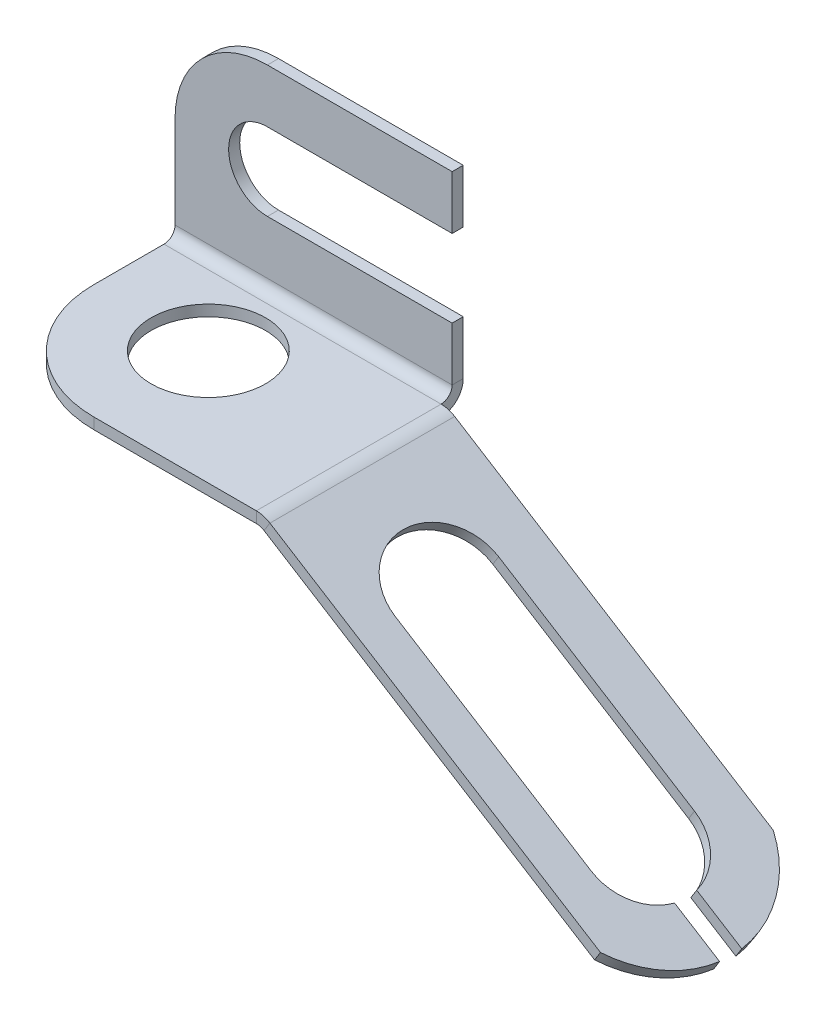
ISO-10303-21;
HEADER;
FILE_DESCRIPTION(('STEP AP214'),'2;1');
FILE_NAME('part.step','',(''),(''),'','','');
FILE_SCHEMA(('AUTOMOTIVE_DESIGN { 1 0 10303 214 1 1 1 1 }'));
ENDSEC;
DATA;
#1=APPLICATION_CONTEXT('core data for automotive mechanical design processes');
#2=APPLICATION_PROTOCOL_DEFINITION('international standard','automotive_design',2000,#1);
#3=PRODUCT_CONTEXT('',#1,'mechanical');
#4=PRODUCT('Part','Part','',(#3));
#5=PRODUCT_RELATED_PRODUCT_CATEGORY('part','',(#4));
#6=PRODUCT_DEFINITION_FORMATION('','',#4);
#7=PRODUCT_DEFINITION_CONTEXT('part definition',#1,'design');
#8=PRODUCT_DEFINITION('design','',#6,#7);
#9=PRODUCT_DEFINITION_SHAPE('','',#8);
#10=(LENGTH_UNIT() NAMED_UNIT(*) SI_UNIT(.MILLI.,.METRE.));
#11=(NAMED_UNIT(*) PLANE_ANGLE_UNIT() SI_UNIT($,.RADIAN.));
#12=(NAMED_UNIT(*) SI_UNIT($,.STERADIAN.) SOLID_ANGLE_UNIT());
#13=UNCERTAINTY_MEASURE_WITH_UNIT(LENGTH_MEASURE(1.E-05),#10,'distance_accuracy_value','');
#14=(GEOMETRIC_REPRESENTATION_CONTEXT(3) GLOBAL_UNCERTAINTY_ASSIGNED_CONTEXT((#13)) GLOBAL_UNIT_ASSIGNED_CONTEXT((#10,
#11,#12)) REPRESENTATION_CONTEXT('',''));
#15=CARTESIAN_POINT('',(0.,0.,0.));
#16=DIRECTION('',(0.,0.,1.));
#17=DIRECTION('',(1.,0.,0.));
#18=AXIS2_PLACEMENT_3D('',#15,#16,#17);
#19=CARTESIAN_POINT('',(0.,0.,0.002000000000002));
#20=DIRECTION('',(0.,-1.,0.));
#21=DIRECTION('',(0.,0.,-1.));
#22=AXIS2_PLACEMENT_3D('',#19,#20,#21);
#23=PLANE('',#22);
#24=CARTESIAN_POINT('',(0.,0.,0.));
#25=DIRECTION('',(0.,1.,0.));
#26=DIRECTION('',(0.,0.,1.));
#27=AXIS2_PLACEMENT_3D('',#24,#25,#26);
#28=CIRCLE('',#27,7.874);
#29=CARTESIAN_POINT('',(0.,0.,7.874));
#30=VERTEX_POINT('',#29);
#31=EDGE_CURVE('E347',#30,#30,#28,.T.);
#32=ORIENTED_EDGE('',*,*,#31,.F.);
#33=EDGE_LOOP('',(#32));
#34=FACE_BOUND('',#33,.T.);
#35=DIRECTION('',(1.,0.,0.));
#36=VECTOR('',#35,1.);
#37=CARTESIAN_POINT('',(0.,0.,15.75));
#38=LINE('',#37,#36);
#39=CARTESIAN_POINT('',(0.,0.,15.75));
#40=VERTEX_POINT('',#39);
#41=CARTESIAN_POINT('',(22.352,0.,15.75));
#42=VERTEX_POINT('',#41);
#43=EDGE_CURVE('E54',#40,#42,#38,.T.);
#44=ORIENTED_EDGE('',*,*,#43,.T.);
#45=DIRECTION('',(0.,0.,-1.));
#46=VECTOR('',#45,1.);
#47=CARTESIAN_POINT('',(22.352,0.,0.002000000000002));
#48=LINE('',#47,#46);
#49=CARTESIAN_POINT('',(22.352,0.,-9.65312139112702));
#50=VERTEX_POINT('',#49);
#51=EDGE_CURVE('E58',#42,#50,#48,.T.);
#52=ORIENTED_EDGE('',*,*,#51,.T.);
#53=DIRECTION('',(1.,0.,0.));
#54=VECTOR('',#53,1.);
#55=CARTESIAN_POINT('',(0.,0.,-9.65312139112702));
#56=LINE('',#55,#54);
#57=CARTESIAN_POINT('',(-15.748,0.,-9.65312139112702));
#58=VERTEX_POINT('',#57);
#59=EDGE_CURVE('E328',#58,#50,#56,.T.);
#60=ORIENTED_EDGE('',*,*,#59,.F.);
#61=DIRECTION('',(0.,0.,1.));
#62=VECTOR('',#61,1.);
#63=CARTESIAN_POINT('',(-15.748,0.,-25.94));
#64=LINE('',#63,#62);
#65=CARTESIAN_POINT('',(-15.748,0.,0.00200000000000489));
#66=VERTEX_POINT('',#65);
#67=EDGE_CURVE('E342',#58,#66,#64,.T.);
#68=ORIENTED_EDGE('',*,*,#67,.T.);
#69=CARTESIAN_POINT('',(0.,0.,0.002000000000002));
#70=DIRECTION('',(0.,1.,0.));
#71=DIRECTION('',(0.,0.,-1.));
#72=AXIS2_PLACEMENT_3D('',#69,#70,#71);
#73=CIRCLE('',#72,15.748);
#74=EDGE_CURVE('E339',#66,#40,#73,.T.);
#75=ORIENTED_EDGE('',*,*,#74,.T.);
#76=EDGE_LOOP('',(#44,#52,#60,#68,#75));
#77=FACE_BOUND('',#76,.T.);
#78=ADVANCED_FACE('F51',(#34,#77),#23,.F.);
#79=CARTESIAN_POINT('',(0.,-11.719678608873,-11.1731213911271));
#80=DIRECTION('',(0.,0.,-1.));
#81=DIRECTION('',(0.,1.,0.));
#82=AXIS2_PLACEMENT_3D('',#79,#80,#81);
#83=PLANE('',#82);
#84=DIRECTION('',(0.,-1.,0.));
#85=VECTOR('',#84,1.);
#86=CARTESIAN_POINT('',(-15.748,14.222321391127,-11.173121391127));
#87=LINE('',#86,#85);
#88=CARTESIAN_POINT('',(-15.748,14.222321391127,-11.173121391127));
#89=VERTEX_POINT('',#88);
#90=CARTESIAN_POINT('',(-15.748,1.52,-11.173121391127));
#91=VERTEX_POINT('',#90);
#92=EDGE_CURVE('E398',#89,#91,#87,.T.);
#93=ORIENTED_EDGE('',*,*,#92,.T.);
#94=DIRECTION('',(1.,0.,0.));
#95=VECTOR('',#94,1.);
#96=CARTESIAN_POINT('',(0.,1.52,-11.173121391127));
#97=LINE('',#96,#95);
#98=CARTESIAN_POINT('',(22.352,1.52,-11.173121391127));
#99=VERTEX_POINT('',#98);
#100=EDGE_CURVE('E420',#91,#99,#97,.T.);
#101=ORIENTED_EDGE('',*,*,#100,.T.);
#102=DIRECTION('',(0.,1.,0.));
#103=VECTOR('',#102,1.);
#104=CARTESIAN_POINT('',(22.352,8.88832139112702,-11.173121391127));
#105=LINE('',#104,#103);
#106=CARTESIAN_POINT('',(22.352,8.88832139112702,-11.173121391127));
#107=VERTEX_POINT('',#106);
#108=EDGE_CURVE('E331',#99,#107,#105,.T.);
#109=ORIENTED_EDGE('',*,*,#108,.T.);
#110=DIRECTION('',(-1.,0.,0.));
#111=VECTOR('',#110,1.);
#112=CARTESIAN_POINT('',(22.352,8.88832139112702,-11.173121391127));
#113=LINE('',#112,#111);
#114=CARTESIAN_POINT('',(-3.04799999999999,8.88832139112702,-11.173121391127));
#115=VERTEX_POINT('',#114);
#116=EDGE_CURVE('E377',#107,#115,#113,.T.);
#117=ORIENTED_EDGE('',*,*,#116,.T.);
#118=CARTESIAN_POINT('',(-3.048,14.222321391127,-11.173121391127));
#119=DIRECTION('',(0.,0.,-1.));
#120=DIRECTION('',(0.,1.,0.));
#121=AXIS2_PLACEMENT_3D('',#118,#119,#120);
#122=CIRCLE('',#121,5.334);
#123=CARTESIAN_POINT('',(-3.048,19.556321391127,-11.173121391127));
#124=VERTEX_POINT('',#123);
#125=EDGE_CURVE('E382',#115,#124,#122,.T.);
#126=ORIENTED_EDGE('',*,*,#125,.T.);
#127=DIRECTION('',(1.,0.,0.));
#128=VECTOR('',#127,1.);
#129=CARTESIAN_POINT('',(-3.048,19.556321391127,-11.173121391127));
#130=LINE('',#129,#128);
#131=CARTESIAN_POINT('',(22.352,19.556321391127,-11.173121391127));
#132=VERTEX_POINT('',#131);
#133=EDGE_CURVE('E381',#124,#132,#130,.T.);
#134=ORIENTED_EDGE('',*,*,#133,.T.);
#135=DIRECTION('',(0.,1.,0.));
#136=VECTOR('',#135,1.);
#137=CARTESIAN_POINT('',(22.352,19.556321391127,-11.173121391127));
#138=LINE('',#137,#136);
#139=CARTESIAN_POINT('',(22.352,26.922321391127,-11.1731213911269));
#140=VERTEX_POINT('',#139);
#141=EDGE_CURVE('E390',#132,#140,#138,.T.);
#142=ORIENTED_EDGE('',*,*,#141,.T.);
#143=DIRECTION('',(-1.,0.,0.));
#144=VECTOR('',#143,1.);
#145=CARTESIAN_POINT('',(22.352,26.922321391127,-11.1731213911269));
#146=LINE('',#145,#144);
#147=CARTESIAN_POINT('',(-3.048,26.922321391127,-11.1731213911269));
#148=VERTEX_POINT('',#147);
#149=EDGE_CURVE('E388',#140,#148,#146,.T.);
#150=ORIENTED_EDGE('',*,*,#149,.T.);
#151=CARTESIAN_POINT('',(-3.048,14.222321391127,-11.173121391127));
#152=DIRECTION('',(0.,0.,1.));
#153=DIRECTION('',(0.,-1.,0.));
#154=AXIS2_PLACEMENT_3D('',#151,#152,#153);
#155=CIRCLE('',#154,12.7);
#156=EDGE_CURVE('E392',#148,#89,#155,.T.);
#157=ORIENTED_EDGE('',*,*,#156,.T.);
#158=EDGE_LOOP('',(#93,#101,#109,#117,#126,#134,#142,#150,#157));
#159=FACE_BOUND('',#158,.T.);
#160=ADVANCED_FACE('F518',(#159),#83,.F.);
#161=CARTESIAN_POINT('',(22.352,8.88832139112703,-12.697121391127));
#162=DIRECTION('',(1.,0.,0.));
#163=DIRECTION('',(0.,1.,0.));
#164=AXIS2_PLACEMENT_3D('',#161,#162,#163);
#165=PLANE('',#164);
#166=DIRECTION('',(0.,0.,1.));
#167=VECTOR('',#166,1.);
#168=CARTESIAN_POINT('',(22.352,1.52000000000001,-12.697121391127));
#169=LINE('',#168,#167);
#170=CARTESIAN_POINT('',(22.352,1.52000000000001,-12.697121391127));
#171=VERTEX_POINT('',#170);
#172=EDGE_CURVE('E414',#171,#99,#169,.T.);
#173=ORIENTED_EDGE('',*,*,#172,.F.);
#174=DIRECTION('',(0.,1.,0.));
#175=VECTOR('',#174,1.);
#176=CARTESIAN_POINT('',(22.352,8.88832139112703,-12.697121391127));
#177=LINE('',#176,#175);
#178=CARTESIAN_POINT('',(22.352,8.88832139112703,-12.697121391127));
#179=VERTEX_POINT('',#178);
#180=EDGE_CURVE('E365',#171,#179,#177,.T.);
#181=ORIENTED_EDGE('',*,*,#180,.T.);
#182=DIRECTION('',(0.,0.,1.));
#183=VECTOR('',#182,1.);
#184=CARTESIAN_POINT('',(22.352,8.88832139112703,-12.697121391127));
#185=LINE('',#184,#183);
#186=EDGE_CURVE('E408',#179,#107,#185,.T.);
#187=ORIENTED_EDGE('',*,*,#186,.T.);
#188=ORIENTED_EDGE('',*,*,#108,.F.);
#189=EDGE_LOOP('',(#173,#181,#187,#188));
#190=FACE_BOUND('',#189,.T.);
#191=ADVANCED_FACE('F530',(#190),#165,.T.);
#192=CARTESIAN_POINT('',(-15.748,14.222321391127,-12.697121391127));
#193=DIRECTION('',(-1.,0.,0.));
#194=DIRECTION('',(0.,-1.,0.));
#195=AXIS2_PLACEMENT_3D('',#192,#193,#194);
#196=PLANE('',#195);
#197=DIRECTION('',(0.,0.,-1.));
#198=VECTOR('',#197,1.);
#199=CARTESIAN_POINT('',(-15.748,1.52000000000001,-12.697121391127));
#200=LINE('',#199,#198);
#201=CARTESIAN_POINT('',(-15.748,1.52000000000001,-12.697121391127));
#202=VERTEX_POINT('',#201);
#203=EDGE_CURVE('E419',#91,#202,#200,.T.);
#204=ORIENTED_EDGE('',*,*,#203,.F.);
#205=ORIENTED_EDGE('',*,*,#92,.F.);
#206=DIRECTION('',(0.,0.,1.));
#207=VECTOR('',#206,1.);
#208=CARTESIAN_POINT('',(-15.748,14.222321391127,-12.697121391127));
#209=LINE('',#208,#207);
#210=CARTESIAN_POINT('',(-15.748,14.222321391127,-12.697121391127));
#211=VERTEX_POINT('',#210);
#212=EDGE_CURVE('E400',#211,#89,#209,.T.);
#213=ORIENTED_EDGE('',*,*,#212,.F.);
#214=DIRECTION('',(0.,-1.,0.));
#215=VECTOR('',#214,1.);
#216=CARTESIAN_POINT('',(-15.748,14.222321391127,-12.697121391127));
#217=LINE('',#216,#215);
#218=EDGE_CURVE('E380',#211,#202,#217,.T.);
#219=ORIENTED_EDGE('',*,*,#218,.T.);
#220=EDGE_LOOP('',(#204,#205,#213,#219));
#221=FACE_BOUND('',#220,.T.);
#222=ADVANCED_FACE('F504',(#221),#196,.T.);
#223=CARTESIAN_POINT('',(-3.048,14.222321391127,-12.697121391127));
#224=DIRECTION('',(0.,0.,1.));
#225=DIRECTION('',(0.,-1.,0.));
#226=AXIS2_PLACEMENT_3D('',#223,#224,#225);
#227=CYLINDRICAL_SURFACE('',#226,12.7);
#228=ORIENTED_EDGE('',*,*,#156,.F.);
#229=DIRECTION('',(0.,0.,1.));
#230=VECTOR('',#229,1.);
#231=CARTESIAN_POINT('',(-3.048,26.922321391127,-12.6971213911269));
#232=LINE('',#231,#230);
#233=CARTESIAN_POINT('',(-3.048,26.922321391127,-12.6971213911269));
#234=VERTEX_POINT('',#233);
#235=EDGE_CURVE('E397',#234,#148,#232,.T.);
#236=ORIENTED_EDGE('',*,*,#235,.F.);
#237=CARTESIAN_POINT('',(-3.048,14.222321391127,-12.697121391127));
#238=DIRECTION('',(0.,0.,1.));
#239=DIRECTION('',(0.,-1.,0.));
#240=AXIS2_PLACEMENT_3D('',#237,#238,#239);
#241=CIRCLE('',#240,12.7);
#242=EDGE_CURVE('E372',#234,#211,#241,.T.);
#243=ORIENTED_EDGE('',*,*,#242,.T.);
#244=ORIENTED_EDGE('',*,*,#212,.T.);
#245=EDGE_LOOP('',(#228,#236,#243,#244));
#246=FACE_BOUND('',#245,.T.);
#247=ADVANCED_FACE('F537',(#246),#227,.T.);
#248=CARTESIAN_POINT('',(22.352,26.922321391127,-12.6971213911269));
#249=DIRECTION('',(0.,1.,0.));
#250=DIRECTION('',(-1.,0.,0.));
#251=AXIS2_PLACEMENT_3D('',#248,#249,#250);
#252=PLANE('',#251);
#253=ORIENTED_EDGE('',*,*,#149,.F.);
#254=DIRECTION('',(0.,0.,1.));
#255=VECTOR('',#254,1.);
#256=CARTESIAN_POINT('',(22.352,26.922321391127,-12.6971213911269));
#257=LINE('',#256,#255);
#258=CARTESIAN_POINT('',(22.352,26.922321391127,-12.6971213911269));
#259=VERTEX_POINT('',#258);
#260=EDGE_CURVE('E405',#259,#140,#257,.T.);
#261=ORIENTED_EDGE('',*,*,#260,.F.);
#262=DIRECTION('',(-1.,0.,0.));
#263=VECTOR('',#262,1.);
#264=CARTESIAN_POINT('',(22.352,26.922321391127,-12.6971213911269));
#265=LINE('',#264,#263);
#266=EDGE_CURVE('E371',#259,#234,#265,.T.);
#267=ORIENTED_EDGE('',*,*,#266,.T.);
#268=ORIENTED_EDGE('',*,*,#235,.T.);
#269=EDGE_LOOP('',(#253,#261,#267,#268));
#270=FACE_BOUND('',#269,.T.);
#271=ADVANCED_FACE('F559',(#270),#252,.T.);
#272=CARTESIAN_POINT('',(22.352,19.556321391127,-12.697121391127));
#273=DIRECTION('',(1.,0.,0.));
#274=DIRECTION('',(0.,1.,0.));
#275=AXIS2_PLACEMENT_3D('',#272,#273,#274);
#276=PLANE('',#275);
#277=ORIENTED_EDGE('',*,*,#141,.F.);
#278=DIRECTION('',(0.,0.,1.));
#279=VECTOR('',#278,1.);
#280=CARTESIAN_POINT('',(22.352,19.556321391127,-12.697121391127));
#281=LINE('',#280,#279);
#282=CARTESIAN_POINT('',(22.352,19.556321391127,-12.697121391127));
#283=VERTEX_POINT('',#282);
#284=EDGE_CURVE('E404',#283,#132,#281,.T.);
#285=ORIENTED_EDGE('',*,*,#284,.F.);
#286=DIRECTION('',(0.,1.,0.));
#287=VECTOR('',#286,1.);
#288=CARTESIAN_POINT('',(22.352,19.556321391127,-12.697121391127));
#289=LINE('',#288,#287);
#290=EDGE_CURVE('E368',#283,#259,#289,.T.);
#291=ORIENTED_EDGE('',*,*,#290,.T.);
#292=ORIENTED_EDGE('',*,*,#260,.T.);
#293=EDGE_LOOP('',(#277,#285,#291,#292));
#294=FACE_BOUND('',#293,.T.);
#295=ADVANCED_FACE('F554',(#294),#276,.T.);
#296=CARTESIAN_POINT('',(-3.048,19.556321391127,-12.697121391127));
#297=DIRECTION('',(0.,-1.,0.));
#298=DIRECTION('',(1.,0.,0.));
#299=AXIS2_PLACEMENT_3D('',#296,#297,#298);
#300=PLANE('',#299);
#301=ORIENTED_EDGE('',*,*,#133,.F.);
#302=DIRECTION('',(0.,0.,1.));
#303=VECTOR('',#302,1.);
#304=CARTESIAN_POINT('',(-3.048,19.556321391127,-12.697121391127));
#305=LINE('',#304,#303);
#306=CARTESIAN_POINT('',(-3.048,19.556321391127,-12.697121391127));
#307=VERTEX_POINT('',#306);
#308=EDGE_CURVE('E407',#307,#124,#305,.T.);
#309=ORIENTED_EDGE('',*,*,#308,.F.);
#310=DIRECTION('',(1.,0.,0.));
#311=VECTOR('',#310,1.);
#312=CARTESIAN_POINT('',(-3.048,19.556321391127,-12.697121391127));
#313=LINE('',#312,#311);
#314=EDGE_CURVE('E362',#307,#283,#313,.T.);
#315=ORIENTED_EDGE('',*,*,#314,.T.);
#316=ORIENTED_EDGE('',*,*,#284,.T.);
#317=EDGE_LOOP('',(#301,#309,#315,#316));
#318=FACE_BOUND('',#317,.T.);
#319=ADVANCED_FACE('F553',(#318),#300,.T.);
#320=CARTESIAN_POINT('',(-3.048,14.222321391127,-12.697121391127));
#321=DIRECTION('',(0.,0.,1.));
#322=DIRECTION('',(0.,-1.,0.));
#323=AXIS2_PLACEMENT_3D('',#320,#321,#322);
#324=CYLINDRICAL_SURFACE('',#323,5.334);
#325=ORIENTED_EDGE('',*,*,#125,.F.);
#326=DIRECTION('',(0.,0.,1.));
#327=VECTOR('',#326,1.);
#328=CARTESIAN_POINT('',(-3.04799999999999,8.88832139112703,-12.697121391127));
#329=LINE('',#328,#327);
#330=CARTESIAN_POINT('',(-3.04799999999999,8.88832139112703,-12.697121391127));
#331=VERTEX_POINT('',#330);
#332=EDGE_CURVE('E409',#331,#115,#329,.T.);
#333=ORIENTED_EDGE('',*,*,#332,.F.);
#334=CARTESIAN_POINT('',(-3.048,14.222321391127,-12.697121391127));
#335=DIRECTION('',(0.,0.,-1.));
#336=DIRECTION('',(0.,1.,0.));
#337=AXIS2_PLACEMENT_3D('',#334,#335,#336);
#338=CIRCLE('',#337,5.334);
#339=EDGE_CURVE('E363',#331,#307,#338,.T.);
#340=ORIENTED_EDGE('',*,*,#339,.T.);
#341=ORIENTED_EDGE('',*,*,#308,.T.);
#342=EDGE_LOOP('',(#325,#333,#340,#341));
#343=FACE_BOUND('',#342,.T.);
#344=ADVANCED_FACE('F550',(#343),#324,.F.);
#345=CARTESIAN_POINT('',(22.352,8.88832139112703,-12.697121391127));
#346=DIRECTION('',(0.,1.,0.));
#347=DIRECTION('',(-1.,0.,0.));
#348=AXIS2_PLACEMENT_3D('',#345,#346,#347);
#349=PLANE('',#348);
#350=ORIENTED_EDGE('',*,*,#116,.F.);
#351=ORIENTED_EDGE('',*,*,#186,.F.);
#352=DIRECTION('',(-1.,0.,0.));
#353=VECTOR('',#352,1.);
#354=CARTESIAN_POINT('',(22.352,8.88832139112703,-12.697121391127));
#355=LINE('',#354,#353);
#356=EDGE_CURVE('E356',#179,#331,#355,.T.);
#357=ORIENTED_EDGE('',*,*,#356,.T.);
#358=ORIENTED_EDGE('',*,*,#332,.T.);
#359=EDGE_LOOP('',(#350,#351,#357,#358));
#360=FACE_BOUND('',#359,.T.);
#361=ADVANCED_FACE('F543',(#360),#349,.T.);
#362=CARTESIAN_POINT('',(0.,-11.719678608873,-12.6971213911271));
#363=DIRECTION('',(0.,0.,-1.));
#364=DIRECTION('',(0.,1.,0.));
#365=AXIS2_PLACEMENT_3D('',#362,#363,#364);
#366=PLANE('',#365);
#367=DIRECTION('',(1.,0.,0.));
#368=VECTOR('',#367,1.);
#369=CARTESIAN_POINT('',(0.,1.52000000000001,-12.697121391127));
#370=LINE('',#369,#368);
#371=EDGE_CURVE('E399',#202,#171,#370,.T.);
#372=ORIENTED_EDGE('',*,*,#371,.F.);
#373=ORIENTED_EDGE('',*,*,#218,.F.);
#374=ORIENTED_EDGE('',*,*,#242,.F.);
#375=ORIENTED_EDGE('',*,*,#266,.F.);
#376=ORIENTED_EDGE('',*,*,#290,.F.);
#377=ORIENTED_EDGE('',*,*,#314,.F.);
#378=ORIENTED_EDGE('',*,*,#339,.F.);
#379=ORIENTED_EDGE('',*,*,#356,.F.);
#380=ORIENTED_EDGE('',*,*,#180,.F.);
#381=EDGE_LOOP('',(#372,#373,#374,#375,#376,#377,#378,#379,#380));
#382=FACE_BOUND('',#381,.T.);
#383=ADVANCED_FACE('F499',(#382),#366,.T.);
#384=CARTESIAN_POINT('',(0.,-1.524,0.002000000000002));
#385=DIRECTION('',(0.,1.,0.));
#386=DIRECTION('',(0.,0.,1.));
#387=AXIS2_PLACEMENT_3D('',#384,#385,#386);
#388=CYLINDRICAL_SURFACE('',#387,15.748);
#389=ORIENTED_EDGE('',*,*,#74,.F.);
#390=DIRECTION('',(0.,1.,0.));
#391=VECTOR('',#390,1.);
#392=CARTESIAN_POINT('',(-15.748,-1.524,0.00200000000000489));
#393=LINE('',#392,#391);
#394=CARTESIAN_POINT('',(-15.748,-1.524,0.00200000000000489));
#395=VERTEX_POINT('',#394);
#396=EDGE_CURVE('E326',#395,#66,#393,.T.);
#397=ORIENTED_EDGE('',*,*,#396,.F.);
#398=CARTESIAN_POINT('',(0.,-1.524,0.002000000000002));
#399=DIRECTION('',(0.,1.,0.));
#400=DIRECTION('',(0.,0.,-1.));
#401=AXIS2_PLACEMENT_3D('',#398,#399,#400);
#402=CIRCLE('',#401,15.748);
#403=CARTESIAN_POINT('',(0.,-1.524,15.75));
#404=VERTEX_POINT('',#403);
#405=EDGE_CURVE('E352',#395,#404,#402,.T.);
#406=ORIENTED_EDGE('',*,*,#405,.T.);
#407=DIRECTION('',(0.,1.,0.));
#408=VECTOR('',#407,1.);
#409=CARTESIAN_POINT('',(0.,-1.524,15.75));
#410=LINE('',#409,#408);
#411=EDGE_CURVE('E355',#404,#40,#410,.T.);
#412=ORIENTED_EDGE('',*,*,#411,.T.);
#413=EDGE_LOOP('',(#389,#397,#406,#412));
#414=FACE_BOUND('',#413,.T.);
#415=ADVANCED_FACE('F542',(#414),#388,.T.);
#416=CARTESIAN_POINT('',(0.,-1.524,15.75));
#417=DIRECTION('',(0.,0.,1.));
#418=DIRECTION('',(1.,0.,0.));
#419=AXIS2_PLACEMENT_3D('',#416,#417,#418);
#420=PLANE('',#419);
#421=DIRECTION('',(0.,-1.,0.));
#422=VECTOR('',#421,1.);
#423=CARTESIAN_POINT('',(22.352,-1.524,15.75));
#424=LINE('',#423,#422);
#425=CARTESIAN_POINT('',(22.352,-1.524,15.75));
#426=VERTEX_POINT('',#425);
#427=EDGE_CURVE('E12',#42,#426,#424,.T.);
#428=ORIENTED_EDGE('',*,*,#427,.F.);
#429=ORIENTED_EDGE('',*,*,#43,.F.);
#430=ORIENTED_EDGE('',*,*,#411,.F.);
#431=DIRECTION('',(1.,0.,0.));
#432=VECTOR('',#431,1.);
#433=CARTESIAN_POINT('',(0.,-1.524,15.75));
#434=LINE('',#433,#432);
#435=EDGE_CURVE('E351',#404,#426,#434,.T.);
#436=ORIENTED_EDGE('',*,*,#435,.T.);
#437=EDGE_LOOP('',(#428,#429,#430,#436));
#438=FACE_BOUND('',#437,.T.);
#439=ADVANCED_FACE('F52',(#438),#420,.T.);
#440=CARTESIAN_POINT('',(0.,-1.524,0.));
#441=DIRECTION('',(0.,1.,0.));
#442=DIRECTION('',(0.,0.,1.));
#443=AXIS2_PLACEMENT_3D('',#440,#441,#442);
#444=CYLINDRICAL_SURFACE('',#443,7.874);
#445=CARTESIAN_POINT('',(0.,-1.524,0.));
#446=DIRECTION('',(0.,1.,0.));
#447=DIRECTION('',(0.,0.,1.));
#448=AXIS2_PLACEMENT_3D('',#445,#446,#447);
#449=CIRCLE('',#448,7.874);
#450=CARTESIAN_POINT('',(0.,-1.524,7.874));
#451=VERTEX_POINT('',#450);
#452=EDGE_CURVE('E343',#451,#451,#449,.T.);
#453=CARTESIAN_POINT('',(0.,-1.524,7.874));
#454=CARTESIAN_POINT('',(0.,-1.508125,7.874));
#455=CARTESIAN_POINT('',(0.,-1.49225,7.874));
#456=CARTESIAN_POINT('',(0.,-1.4605,7.874));
#457=CARTESIAN_POINT('',(0.,-1.444625,7.874));
#458=CARTESIAN_POINT('',(0.,-1.412875,7.874));
#459=CARTESIAN_POINT('',(0.,-1.397,7.874));
#460=CARTESIAN_POINT('',(0.,-1.36525,7.874));
#461=CARTESIAN_POINT('',(0.,-1.349375,7.874));
#462=CARTESIAN_POINT('',(0.,-1.317625,7.874));
#463=CARTESIAN_POINT('',(0.,-1.30175,7.874));
#464=CARTESIAN_POINT('',(0.,-1.27,7.874));
#465=CARTESIAN_POINT('',(0.,-1.254125,7.874));
#466=CARTESIAN_POINT('',(0.,-1.222375,7.874));
#467=CARTESIAN_POINT('',(0.,-1.2065,7.874));
#468=CARTESIAN_POINT('',(0.,-1.17475,7.874));
#469=CARTESIAN_POINT('',(0.,-1.158875,7.874));
#470=CARTESIAN_POINT('',(0.,-1.127125,7.874));
#471=CARTESIAN_POINT('',(0.,-1.11125,7.874));
#472=CARTESIAN_POINT('',(0.,-1.0795,7.874));
#473=CARTESIAN_POINT('',(0.,-1.063625,7.874));
#474=CARTESIAN_POINT('',(0.,-1.031875,7.874));
#475=CARTESIAN_POINT('',(0.,-1.016,7.874));
#476=CARTESIAN_POINT('',(0.,-0.98425,7.874));
#477=CARTESIAN_POINT('',(0.,-0.968375,7.874));
#478=CARTESIAN_POINT('',(0.,-0.936625,7.874));
#479=CARTESIAN_POINT('',(0.,-0.92075,7.874));
#480=CARTESIAN_POINT('',(0.,-0.889,7.874));
#481=CARTESIAN_POINT('',(0.,-0.873125,7.874));
#482=CARTESIAN_POINT('',(0.,-0.841375,7.874));
#483=CARTESIAN_POINT('',(0.,-0.8255,7.874));
#484=CARTESIAN_POINT('',(0.,-0.79375,7.874));
#485=CARTESIAN_POINT('',(0.,-0.777875,7.874));
#486=CARTESIAN_POINT('',(0.,-0.746125,7.874));
#487=CARTESIAN_POINT('',(0.,-0.73025,7.874));
#488=CARTESIAN_POINT('',(0.,-0.6985,7.874));
#489=CARTESIAN_POINT('',(0.,-0.682625,7.874));
#490=CARTESIAN_POINT('',(0.,-0.650875,7.874));
#491=CARTESIAN_POINT('',(0.,-0.635,7.874));
#492=CARTESIAN_POINT('',(0.,-0.60325,7.874));
#493=CARTESIAN_POINT('',(0.,-0.587375,7.874));
#494=CARTESIAN_POINT('',(0.,-0.555625,7.874));
#495=CARTESIAN_POINT('',(0.,-0.53975,7.874));
#496=CARTESIAN_POINT('',(0.,-0.508,7.874));
#497=CARTESIAN_POINT('',(0.,-0.492125,7.874));
#498=CARTESIAN_POINT('',(0.,-0.460375,7.874));
#499=CARTESIAN_POINT('',(0.,-0.4445,7.874));
#500=CARTESIAN_POINT('',(0.,-0.41275,7.874));
#501=CARTESIAN_POINT('',(0.,-0.396875,7.874));
#502=CARTESIAN_POINT('',(0.,-0.365125,7.874));
#503=CARTESIAN_POINT('',(0.,-0.34925,7.874));
#504=CARTESIAN_POINT('',(0.,-0.3175,7.874));
#505=CARTESIAN_POINT('',(0.,-0.301625,7.874));
#506=CARTESIAN_POINT('',(0.,-0.269875,7.874));
#507=CARTESIAN_POINT('',(0.,-0.254,7.874));
#508=CARTESIAN_POINT('',(0.,-0.22225,7.874));
#509=CARTESIAN_POINT('',(0.,-0.206375,7.874));
#510=CARTESIAN_POINT('',(0.,-0.174625,7.874));
#511=CARTESIAN_POINT('',(0.,-0.15875,7.874));
#512=CARTESIAN_POINT('',(0.,-0.127,7.874));
#513=CARTESIAN_POINT('',(0.,-0.111125,7.874));
#514=CARTESIAN_POINT('',(0.,-0.079375,7.874));
#515=CARTESIAN_POINT('',(0.,-0.0635,7.874));
#516=CARTESIAN_POINT('',(0.,-0.0317499999999999,7.874));
#517=CARTESIAN_POINT('',(0.,-0.015875,7.874));
#518=CARTESIAN_POINT('',(0.,0.,7.874));
#519=B_SPLINE_CURVE_WITH_KNOTS('',3,(#453,#454,#455,#456,#457,#458,#459,#460,#461,#462,#463,
#464,#465,#466,#467,#468,#469,#470,#471,#472,#473,#474,#475,#476,#477,#478,#479,#480,#481,#482,
#483,#484,#485,#486,#487,#488,#489,#490,#491,#492,#493,#494,#495,#496,#497,#498,#499,#500,#501,
#502,#503,#504,#505,#506,#507,#508,#509,#510,#511,#512,#513,#514,#515,#516,#517,#518),
.UNSPECIFIED.,.F.,.F.,(4,2,2,2,2,2,2,2,2,2,2,2,2,2,2,2,2,2,2,2,2,2,2,2,2,2,2,2,2,2,2,2,4),(0.,
0.0476250000000001,0.0952500000000001,0.142875,0.1905,0.238125,0.28575,0.333375,0.381,0.428625,
0.47625,0.523875,0.5715,0.619125,0.66675,0.714375,0.762,0.809625,0.85725,0.904875,0.9525,
1.000125,1.04775,1.095375,1.143,1.190625,1.23825,1.285875,1.3335,1.381125,1.42875,1.476375,
1.524),.UNSPECIFIED.);
#520=EDGE_CURVE('BSEAM534',#451,#30,#519,.T.);
#521=ORIENTED_EDGE('',*,*,#452,.F.);
#522=ORIENTED_EDGE('',*,*,#31,.T.);
#523=ORIENTED_EDGE('',*,*,#520,.T.);
#524=ORIENTED_EDGE('',*,*,#520,.F.);
#525=EDGE_LOOP('',(#521,#523,#522,#524));
#526=FACE_BOUND('',#525,.T.);
#527=ADVANCED_FACE('F534',(#526),#444,.F.);
#528=CARTESIAN_POINT('',(0.,-1.524,0.002000000000002));
#529=DIRECTION('',(0.,-1.,0.));
#530=DIRECTION('',(0.,0.,-1.));
#531=AXIS2_PLACEMENT_3D('',#528,#529,#530);
#532=PLANE('',#531);
#533=DIRECTION('',(0.,0.,-1.));
#534=VECTOR('',#533,1.);
#535=CARTESIAN_POINT('',(22.352,-1.524,0.002000000000002));
#536=LINE('',#535,#534);
#537=CARTESIAN_POINT('',(22.352,-1.524,-9.65312139112702));
#538=VERTEX_POINT('',#537);
#539=EDGE_CURVE('E421',#426,#538,#536,.T.);
#540=ORIENTED_EDGE('',*,*,#539,.F.);
#541=ORIENTED_EDGE('',*,*,#435,.F.);
#542=ORIENTED_EDGE('',*,*,#405,.F.);
#543=DIRECTION('',(0.,0.,1.));
#544=VECTOR('',#543,1.);
#545=CARTESIAN_POINT('',(-15.748,-1.524,-25.94));
#546=LINE('',#545,#544);
#547=CARTESIAN_POINT('',(-15.748,-1.524,-9.65312139112702));
#548=VERTEX_POINT('',#547);
#549=EDGE_CURVE('E334',#548,#395,#546,.T.);
#550=ORIENTED_EDGE('',*,*,#549,.F.);
#551=DIRECTION('',(1.,0.,0.));
#552=VECTOR('',#551,1.);
#553=CARTESIAN_POINT('',(0.,-1.524,-9.65312139112702));
#554=LINE('',#553,#552);
#555=EDGE_CURVE('E344',#548,#538,#554,.T.);
#556=ORIENTED_EDGE('',*,*,#555,.T.);
#557=EDGE_LOOP('',(#540,#541,#542,#550,#556));
#558=FACE_BOUND('',#557,.T.);
#559=ORIENTED_EDGE('',*,*,#452,.T.);
#560=EDGE_LOOP('',(#559));
#561=FACE_BOUND('',#560,.T.);
#562=ADVANCED_FACE('F439',(#558,#561),#532,.T.);
#563=CARTESIAN_POINT('',(-15.748,-1.524,-25.94));
#564=DIRECTION('',(-1.,0.,0.));
#565=DIRECTION('',(0.,0.,1.));
#566=AXIS2_PLACEMENT_3D('',#563,#564,#565);
#567=PLANE('',#566);
#568=ORIENTED_EDGE('',*,*,#67,.F.);
#569=DIRECTION('',(0.,-1.,0.));
#570=VECTOR('',#569,1.);
#571=CARTESIAN_POINT('',(-15.748,-1.524,-9.65312139112702));
#572=LINE('',#571,#570);
#573=EDGE_CURVE('E337',#58,#548,#572,.T.);
#574=ORIENTED_EDGE('',*,*,#573,.T.);
#575=ORIENTED_EDGE('',*,*,#549,.T.);
#576=ORIENTED_EDGE('',*,*,#396,.T.);
#577=EDGE_LOOP('',(#568,#574,#575,#576));
#578=FACE_BOUND('',#577,.T.);
#579=ADVANCED_FACE('F517',(#578),#567,.T.);
#580=CARTESIAN_POINT('',(-15.748,1.52,-9.65312139112702));
#581=DIRECTION('',(-1.,0.,0.));
#582=DIRECTION('',(0.,0.,1.));
#583=AXIS2_PLACEMENT_3D('',#580,#581,#582);
#584=PLANE('',#583);
#585=ORIENTED_EDGE('',*,*,#573,.F.);
#586=CARTESIAN_POINT('',(-15.748,1.52,-9.65312139112702));
#587=DIRECTION('',(1.,0.,0.));
#588=DIRECTION('',(0.,0.,-1.));
#589=AXIS2_PLACEMENT_3D('',#586,#587,#588);
#590=CIRCLE('',#589,1.52);
#591=EDGE_CURVE('E314',#58,#91,#590,.T.);
#592=ORIENTED_EDGE('',*,*,#591,.T.);
#593=ORIENTED_EDGE('',*,*,#203,.T.);
#594=CARTESIAN_POINT('',(-15.748,1.52,-9.65312139112702));
#595=DIRECTION('',(1.,0.,0.));
#596=DIRECTION('',(0.,0.,1.));
#597=AXIS2_PLACEMENT_3D('',#594,#595,#596);
#598=CIRCLE('',#597,3.044);
#599=EDGE_CURVE('E318',#548,#202,#598,.T.);
#600=ORIENTED_EDGE('',*,*,#599,.F.);
#601=EDGE_LOOP('',(#585,#592,#593,#600));
#602=FACE_BOUND('',#601,.T.);
#603=ADVANCED_FACE('F508',(#602),#584,.T.);
#604=CARTESIAN_POINT('',(22.352,1.52,-9.65312139112702));
#605=DIRECTION('',(1.,0.,0.));
#606=DIRECTION('',(0.,0.,-1.));
#607=AXIS2_PLACEMENT_3D('',#604,#605,#606);
#608=PLANE('',#607);
#609=CARTESIAN_POINT('',(22.352,1.52,-9.65312139112702));
#610=DIRECTION('',(1.,0.,0.));
#611=DIRECTION('',(0.,0.,-1.));
#612=AXIS2_PLACEMENT_3D('',#609,#610,#611);
#613=CIRCLE('',#612,1.52);
#614=EDGE_CURVE('E72',#99,#50,#613,.F.);
#615=ORIENTED_EDGE('',*,*,#614,.T.);
#616=DIRECTION('',(0.,1.,0.));
#617=VECTOR('',#616,1.);
#618=CARTESIAN_POINT('',(22.352,-1.524,-9.65312139112702));
#619=LINE('',#618,#617);
#620=EDGE_CURVE('E431',#538,#50,#619,.T.);
#621=ORIENTED_EDGE('',*,*,#620,.F.);
#622=CARTESIAN_POINT('',(22.352,1.52,-9.65312139112702));
#623=DIRECTION('',(-1.,0.,0.));
#624=DIRECTION('',(0.,0.,-1.));
#625=AXIS2_PLACEMENT_3D('',#622,#623,#624);
#626=CIRCLE('',#625,3.044);
#627=EDGE_CURVE('E324',#171,#538,#626,.T.);
#628=ORIENTED_EDGE('',*,*,#627,.F.);
#629=ORIENTED_EDGE('',*,*,#172,.T.);
#630=EDGE_LOOP('',(#615,#621,#628,#629));
#631=FACE_BOUND('',#630,.T.);
#632=ADVANCED_FACE('F491',(#631),#608,.T.);
#633=CARTESIAN_POINT('',(-34.9965851755296,1.52,-9.65312139112702));
#634=DIRECTION('',(1.,0.,0.));
#635=DIRECTION('',(0.,0.,-1.));
#636=AXIS2_PLACEMENT_3D('',#633,#634,#635);
#637=CYLINDRICAL_SURFACE('',#636,3.044);
#638=ORIENTED_EDGE('',*,*,#371,.T.);
#639=ORIENTED_EDGE('',*,*,#627,.T.);
#640=ORIENTED_EDGE('',*,*,#555,.F.);
#641=ORIENTED_EDGE('',*,*,#599,.T.);
#642=EDGE_LOOP('',(#638,#639,#640,#641));
#643=FACE_BOUND('',#642,.T.);
#644=ADVANCED_FACE('F492',(#643),#637,.T.);
#645=CARTESIAN_POINT('',(-34.9965851755296,1.52,-9.65312139112702));
#646=DIRECTION('',(1.,0.,0.));
#647=DIRECTION('',(0.,0.,-1.));
#648=AXIS2_PLACEMENT_3D('',#645,#646,#647);
#649=CYLINDRICAL_SURFACE('',#648,1.52);
#650=ORIENTED_EDGE('',*,*,#100,.F.);
#651=ORIENTED_EDGE('',*,*,#591,.F.);
#652=ORIENTED_EDGE('',*,*,#59,.T.);
#653=ORIENTED_EDGE('',*,*,#614,.F.);
#654=EDGE_LOOP('',(#650,#651,#652,#653));
#655=FACE_BOUND('',#654,.T.);
#656=ADVANCED_FACE('F514',(#655),#649,.F.);
#657=CARTESIAN_POINT('',(22.352,-3.524,15.75));
#658=DIRECTION('',(0.,0.,-1.));
#659=DIRECTION('',(-1.,0.,0.));
#660=AXIS2_PLACEMENT_3D('',#657,#658,#659);
#661=PLANE('',#660);
#662=DIRECTION('',(-0.529919264233206,-0.848048096156425,0.));
#663=VECTOR('',#662,1.);
#664=CARTESIAN_POINT('',(23.4118385284664,-1.82790380768715,15.75));
#665=LINE('',#664,#663);
#666=CARTESIAN_POINT('',(24.2194354871578,-0.535478509144757,15.75));
#667=VERTEX_POINT('',#666);
#668=CARTESIAN_POINT('',(23.4118385284664,-1.82790380768715,15.75));
#669=VERTEX_POINT('',#668);
#670=EDGE_CURVE('E232',#667,#669,#665,.T.);
#671=ORIENTED_EDGE('',*,*,#670,.F.);
#672=CARTESIAN_POINT('',(22.352,-3.524,15.75));
#673=DIRECTION('',(0.,0.,1.));
#674=DIRECTION('',(1.,0.,0.));
#675=AXIS2_PLACEMENT_3D('',#672,#673,#674);
#676=CIRCLE('',#675,3.524);
#677=EDGE_CURVE('E250',#667,#42,#676,.T.);
#678=ORIENTED_EDGE('',*,*,#677,.T.);
#679=ORIENTED_EDGE('',*,*,#427,.T.);
#680=CARTESIAN_POINT('',(22.352,-3.524,15.75));
#681=DIRECTION('',(0.,0.,1.));
#682=DIRECTION('',(-1.,0.,0.));
#683=AXIS2_PLACEMENT_3D('',#680,#681,#682);
#684=CIRCLE('',#683,2.);
#685=EDGE_CURVE('E308',#669,#426,#684,.T.);
#686=ORIENTED_EDGE('',*,*,#685,.F.);
#687=EDGE_LOOP('',(#671,#678,#679,#686));
#688=FACE_BOUND('',#687,.T.);
#689=ADVANCED_FACE('F450',(#688),#661,.F.);
#690=CARTESIAN_POINT('',(22.352,-3.524,-9.65312139112702));
#691=DIRECTION('',(0.,0.,1.));
#692=DIRECTION('',(1.,0.,0.));
#693=AXIS2_PLACEMENT_3D('',#690,#691,#692);
#694=PLANE('',#693);
#695=CARTESIAN_POINT('',(22.352,-3.524,-9.65312139112701));
#696=DIRECTION('',(0.,0.,1.));
#697=DIRECTION('',(1.,0.,0.));
#698=AXIS2_PLACEMENT_3D('',#695,#696,#697);
#699=CIRCLE('',#698,3.524);
#700=CARTESIAN_POINT('',(24.2194354871578,-0.535478509144757,-9.65312139112702));
#701=VERTEX_POINT('',#700);
#702=EDGE_CURVE('E315',#50,#701,#699,.F.);
#703=ORIENTED_EDGE('',*,*,#702,.T.);
#704=DIRECTION('',(0.529919264233206,0.848048096156425,0.));
#705=VECTOR('',#704,1.);
#706=CARTESIAN_POINT('',(23.4118385284664,-1.82790380768715,-9.65312139112702));
#707=LINE('',#706,#705);
#708=CARTESIAN_POINT('',(23.4118385284664,-1.82790380768715,-9.65312139112702));
#709=VERTEX_POINT('',#708);
#710=EDGE_CURVE('E466',#709,#701,#707,.T.);
#711=ORIENTED_EDGE('',*,*,#710,.F.);
#712=CARTESIAN_POINT('',(22.352,-3.524,-9.65312139112702));
#713=DIRECTION('',(0.,0.,-1.));
#714=DIRECTION('',(1.,0.,0.));
#715=AXIS2_PLACEMENT_3D('',#712,#713,#714);
#716=CIRCLE('',#715,2.);
#717=EDGE_CURVE('E311',#538,#709,#716,.T.);
#718=ORIENTED_EDGE('',*,*,#717,.F.);
#719=ORIENTED_EDGE('',*,*,#620,.T.);
#720=EDGE_LOOP('',(#703,#711,#718,#719));
#721=FACE_BOUND('',#720,.T.);
#722=ADVANCED_FACE('F493',(#721),#694,.F.);
#723=CARTESIAN_POINT('',(22.352,-3.524,-22.4470650422621));
#724=DIRECTION('',(0.,0.,1.));
#725=DIRECTION('',(1.,0.,0.));
#726=AXIS2_PLACEMENT_3D('',#723,#724,#725);
#727=CYLINDRICAL_SURFACE('',#726,2.);
#728=ORIENTED_EDGE('',*,*,#539,.T.);
#729=ORIENTED_EDGE('',*,*,#717,.T.);
#730=DIRECTION('',(0.,0.,-1.));
#731=VECTOR('',#730,1.);
#732=CARTESIAN_POINT('',(23.4118385284664,-1.82790380768715,0.002000000000002));
#733=LINE('',#732,#731);
#734=EDGE_CURVE('E269',#669,#709,#733,.T.);
#735=ORIENTED_EDGE('',*,*,#734,.F.);
#736=ORIENTED_EDGE('',*,*,#685,.T.);
#737=EDGE_LOOP('',(#728,#729,#735,#736));
#738=FACE_BOUND('',#737,.T.);
#739=ADVANCED_FACE('F446',(#738),#727,.F.);
#740=CARTESIAN_POINT('',(22.352,-3.524,-22.4470650422621));
#741=DIRECTION('',(0.,0.,1.));
#742=DIRECTION('',(1.,0.,0.));
#743=AXIS2_PLACEMENT_3D('',#740,#741,#742);
#744=CYLINDRICAL_SURFACE('',#743,3.524);
#745=ORIENTED_EDGE('',*,*,#51,.F.);
#746=ORIENTED_EDGE('',*,*,#677,.F.);
#747=DIRECTION('',(0.,0.,-1.));
#748=VECTOR('',#747,1.);
#749=CARTESIAN_POINT('',(24.2194354871578,-0.535478509144757,0.002000000000002));
#750=LINE('',#749,#748);
#751=EDGE_CURVE('E259',#667,#701,#750,.T.);
#752=ORIENTED_EDGE('',*,*,#751,.T.);
#753=ORIENTED_EDGE('',*,*,#702,.F.);
#754=EDGE_LOOP('',(#745,#746,#752,#753));
#755=FACE_BOUND('',#754,.T.);
#756=ADVANCED_FACE('F489',(#755),#744,.T.);
#757=CARTESIAN_POINT('',(62.4767570027001,-26.2383740970723,3.55));
#758=DIRECTION('',(0.529919264233206,0.848048096156425,0.));
#759=DIRECTION('',(0.,0.,1.));
#760=AXIS2_PLACEMENT_3D('',#757,#758,#759);
#761=CYLINDRICAL_SURFACE('',#760,14.3346893367871);
#762=DIRECTION('',(0.529919264233206,0.848048096156425,0.));
#763=VECTOR('',#762,1.);
#764=CARTESIAN_POINT('',(70.0727696433476,-40.9796057398259,5.074));
#765=LINE('',#764,#763);
#766=CARTESIAN_POINT('',(74.5643653269883,-33.7915500768041,5.074));
#767=VERTEX_POINT('',#766);
#768=CARTESIAN_POINT('',(75.3719622856797,-32.4991247782617,5.074));
#769=VERTEX_POINT('',#768);
#770=EDGE_CURVE('E254',#767,#769,#765,.T.);
#771=ORIENTED_EDGE('',*,*,#770,.T.);
#772=CARTESIAN_POINT('',(63.2843539613915,-24.9459487985299,3.55));
#773=DIRECTION('',(0.529919264233206,0.848048096156425,0.));
#774=DIRECTION('',(0.,0.,1.));
#775=AXIS2_PLACEMENT_3D('',#772,#773,#774);
#776=CIRCLE('',#775,14.3346893367871);
#777=CARTESIAN_POINT('',(69.6669128063745,-28.9342142075176,15.75));
#778=VERTEX_POINT('',#777);
#779=EDGE_CURVE('E246',#778,#769,#776,.T.);
#780=ORIENTED_EDGE('',*,*,#779,.F.);
#781=DIRECTION('',(0.529919264233206,0.848048096156425,0.));
#782=VECTOR('',#781,1.);
#783=CARTESIAN_POINT('',(68.859315847683,-30.22663950606,15.75));
#784=LINE('',#783,#782);
#785=CARTESIAN_POINT('',(68.859315847683,-30.22663950606,15.75));
#786=VERTEX_POINT('',#785);
#787=EDGE_CURVE('E235',#786,#778,#784,.T.);
#788=ORIENTED_EDGE('',*,*,#787,.F.);
#789=CARTESIAN_POINT('',(62.4767570027001,-26.2383740970723,3.55));
#790=DIRECTION('',(0.529919264233206,0.848048096156425,0.));
#791=DIRECTION('',(0.,0.,1.));
#792=AXIS2_PLACEMENT_3D('',#789,#790,#791);
#793=CIRCLE('',#792,14.3346893367871);
#794=EDGE_CURVE('E242',#786,#767,#793,.T.);
#795=ORIENTED_EDGE('',*,*,#794,.T.);
#796=EDGE_LOOP('',(#771,#780,#788,#795));
#797=FACE_BOUND('',#796,.T.);
#798=ADVANCED_FACE('F243',(#797),#761,.T.);
#799=CARTESIAN_POINT('',(63.8763780343853,-37.1076705309573,5.074));
#800=DIRECTION('',(0.,0.,1.));
#801=DIRECTION('',(0.848048096156425,-0.529919264233206,0.));
#802=AXIS2_PLACEMENT_3D('',#799,#800,#801);
#803=PLANE('',#802);
#804=DIRECTION('',(-0.848048096156425,0.529919264233206,0.));
#805=VECTOR('',#804,1.);
#806=CARTESIAN_POINT('',(3.14807543888309,10.834300701345,5.074));
#807=LINE('',#806,#805);
#808=CARTESIAN_POINT('',(68.367973718026,-29.9196148679354,5.074));
#809=VERTEX_POINT('',#808);
#810=EDGE_CURVE('E255',#767,#809,#807,.T.);
#811=ORIENTED_EDGE('',*,*,#810,.T.);
#812=DIRECTION('',(0.529919264233206,0.848048096156425,0.));
#813=VECTOR('',#812,1.);
#814=CARTESIAN_POINT('',(68.367973718026,-29.9196148679354,5.074));
#815=LINE('',#814,#813);
#816=CARTESIAN_POINT('',(69.1755706767174,-28.627189569393,5.074));
#817=VERTEX_POINT('',#816);
#818=EDGE_CURVE('E285',#817,#809,#815,.F.);
#819=ORIENTED_EDGE('',*,*,#818,.F.);
#820=DIRECTION('',(0.848048096156425,-0.529919264233206,0.));
#821=VECTOR('',#820,1.);
#822=CARTESIAN_POINT('',(69.1755706767174,-28.627189569393,5.074));
#823=LINE('',#822,#821);
#824=EDGE_CURVE('E257',#817,#769,#823,.T.);
#825=ORIENTED_EDGE('',*,*,#824,.T.);
#826=ORIENTED_EDGE('',*,*,#770,.F.);
#827=EDGE_LOOP('',(#811,#819,#825,#826));
#828=FACE_BOUND('',#827,.T.);
#829=ADVANCED_FACE('F617',(#828),#803,.F.);
#830=CARTESIAN_POINT('',(62.4767570027001,-26.2383740970723,3.55));
#831=DIRECTION('',(0.529919264233206,0.848048096156425,0.));
#832=DIRECTION('',(0.,0.,1.));
#833=AXIS2_PLACEMENT_3D('',#830,#831,#832);
#834=CYLINDRICAL_SURFACE('',#833,7.112);
#835=CARTESIAN_POINT('',(63.2843539613915,-24.9459487985299,3.55));
#836=DIRECTION('',(0.529919264233206,0.848048096156425,0.));
#837=DIRECTION('',(0.,0.,1.));
#838=AXIS2_PLACEMENT_3D('',#835,#836,#837);
#839=CIRCLE('',#838,7.112);
#840=CARTESIAN_POINT('',(63.2843539613915,-24.9459487985299,10.662));
#841=VERTEX_POINT('',#840);
#842=EDGE_CURVE('E276',#841,#817,#839,.T.);
#843=ORIENTED_EDGE('',*,*,#842,.T.);
#844=ORIENTED_EDGE('',*,*,#818,.T.);
#845=CARTESIAN_POINT('',(62.4767570027001,-26.2383740970723,3.55));
#846=DIRECTION('',(0.529919264233206,0.848048096156425,0.));
#847=DIRECTION('',(0.,0.,1.));
#848=AXIS2_PLACEMENT_3D('',#845,#846,#847);
#849=CIRCLE('',#848,7.112);
#850=CARTESIAN_POINT('',(62.4767570027001,-26.2383740970723,10.662));
#851=VERTEX_POINT('',#850);
#852=EDGE_CURVE('E458',#851,#809,#849,.T.);
#853=ORIENTED_EDGE('',*,*,#852,.F.);
#854=DIRECTION('',(0.529919264233206,0.848048096156425,0.));
#855=VECTOR('',#854,1.);
#856=CARTESIAN_POINT('',(62.4767570027001,-26.2383740970723,10.662));
#857=LINE('',#856,#855);
#858=EDGE_CURVE('E301',#851,#841,#857,.T.);
#859=ORIENTED_EDGE('',*,*,#858,.T.);
#860=EDGE_LOOP('',(#843,#844,#853,#859));
#861=FACE_BOUND('',#860,.T.);
#862=ADVANCED_FACE('F613',(#861),#834,.F.);
#863=CARTESIAN_POINT('',(35.5512299497336,-9.41343745766802,10.662));
#864=DIRECTION('',(0.,0.,1.));
#865=DIRECTION('',(0.848048096156425,-0.529919264233206,0.));
#866=AXIS2_PLACEMENT_3D('',#863,#864,#865);
#867=PLANE('',#866);
#868=DIRECTION('',(0.848048096156425,-0.529919264233206,0.));
#869=VECTOR('',#868,1.);
#870=CARTESIAN_POINT('',(36.358826908425,-8.12101215912563,10.662));
#871=LINE('',#870,#869);
#872=CARTESIAN_POINT('',(36.358826908425,-8.12101215912563,10.662));
#873=VERTEX_POINT('',#872);
#874=EDGE_CURVE('E296',#873,#841,#871,.T.);
#875=ORIENTED_EDGE('',*,*,#874,.T.);
#876=ORIENTED_EDGE('',*,*,#858,.F.);
#877=DIRECTION('',(0.848048096156425,-0.529919264233206,0.));
#878=VECTOR('',#877,1.);
#879=CARTESIAN_POINT('',(35.5512299497336,-9.41343745766802,10.662));
#880=LINE('',#879,#878);
#881=CARTESIAN_POINT('',(35.5512299497336,-9.41343745766802,10.662));
#882=VERTEX_POINT('',#881);
#883=EDGE_CURVE('E461',#882,#851,#880,.T.);
#884=ORIENTED_EDGE('',*,*,#883,.F.);
#885=DIRECTION('',(0.529919264233206,0.848048096156425,0.));
#886=VECTOR('',#885,1.);
#887=CARTESIAN_POINT('',(35.5512299497336,-9.41343745766802,10.662));
#888=LINE('',#887,#886);
#889=EDGE_CURVE('E294',#882,#873,#888,.T.);
#890=ORIENTED_EDGE('',*,*,#889,.T.);
#891=EDGE_LOOP('',(#875,#876,#884,#890));
#892=FACE_BOUND('',#891,.T.);
#893=ADVANCED_FACE('F608',(#892),#867,.F.);
#894=CARTESIAN_POINT('',(35.5512299497336,-9.41343745766802,3.55));
#895=DIRECTION('',(0.529919264233206,0.848048096156425,0.));
#896=DIRECTION('',(0.,0.,1.));
#897=AXIS2_PLACEMENT_3D('',#894,#895,#896);
#898=CYLINDRICAL_SURFACE('',#897,7.112);
#899=CARTESIAN_POINT('',(36.358826908425,-8.12101215912563,3.55));
#900=DIRECTION('',(0.529919264233206,0.848048096156425,0.));
#901=DIRECTION('',(0.,0.,1.));
#902=AXIS2_PLACEMENT_3D('',#899,#900,#901);
#903=CIRCLE('',#902,7.112);
#904=CARTESIAN_POINT('',(36.358826908425,-8.12101215912563,-3.562));
#905=VERTEX_POINT('',#904);
#906=EDGE_CURVE('E291',#905,#873,#903,.T.);
#907=ORIENTED_EDGE('',*,*,#906,.T.);
#908=ORIENTED_EDGE('',*,*,#889,.F.);
#909=CARTESIAN_POINT('',(35.5512299497336,-9.41343745766802,3.55));
#910=DIRECTION('',(0.529919264233206,0.848048096156425,0.));
#911=DIRECTION('',(0.,0.,1.));
#912=AXIS2_PLACEMENT_3D('',#909,#910,#911);
#913=CIRCLE('',#912,7.112);
#914=CARTESIAN_POINT('',(35.5512299497336,-9.41343745766802,-3.562));
#915=VERTEX_POINT('',#914);
#916=EDGE_CURVE('E456',#915,#882,#913,.T.);
#917=ORIENTED_EDGE('',*,*,#916,.F.);
#918=DIRECTION('',(0.529919264233206,0.848048096156425,0.));
#919=VECTOR('',#918,1.);
#920=CARTESIAN_POINT('',(35.5512299497336,-9.41343745766802,-3.562));
#921=LINE('',#920,#919);
#922=EDGE_CURVE('E293',#915,#905,#921,.T.);
#923=ORIENTED_EDGE('',*,*,#922,.T.);
#924=EDGE_LOOP('',(#907,#908,#917,#923));
#925=FACE_BOUND('',#924,.T.);
#926=ADVANCED_FACE('F603',(#925),#898,.F.);
#927=CARTESIAN_POINT('',(35.5512299497336,-9.41343745766802,-3.562));
#928=DIRECTION('',(0.,0.,-1.));
#929=DIRECTION('',(-0.848048096156425,0.529919264233206,0.));
#930=AXIS2_PLACEMENT_3D('',#927,#928,#929);
#931=PLANE('',#930);
#932=DIRECTION('',(-0.848048096156425,0.529919264233206,0.));
#933=VECTOR('',#932,1.);
#934=CARTESIAN_POINT('',(36.358826908425,-8.12101215912563,-3.562));
#935=LINE('',#934,#933);
#936=CARTESIAN_POINT('',(63.2843539613915,-24.9459487985299,-3.562));
#937=VERTEX_POINT('',#936);
#938=EDGE_CURVE('E288',#937,#905,#935,.T.);
#939=ORIENTED_EDGE('',*,*,#938,.T.);
#940=ORIENTED_EDGE('',*,*,#922,.F.);
#941=DIRECTION('',(-0.848048096156425,0.529919264233206,0.));
#942=VECTOR('',#941,1.);
#943=CARTESIAN_POINT('',(35.5512299497336,-9.41343745766802,-3.562));
#944=LINE('',#943,#942);
#945=CARTESIAN_POINT('',(62.4767570027001,-26.2383740970723,-3.562));
#946=VERTEX_POINT('',#945);
#947=EDGE_CURVE('E451',#946,#915,#944,.T.);
#948=ORIENTED_EDGE('',*,*,#947,.F.);
#949=DIRECTION('',(0.529919264233206,0.848048096156425,0.));
#950=VECTOR('',#949,1.);
#951=CARTESIAN_POINT('',(62.4767570027001,-26.2383740970723,-3.562));
#952=LINE('',#951,#950);
#953=EDGE_CURVE('E284',#946,#937,#952,.T.);
#954=ORIENTED_EDGE('',*,*,#953,.T.);
#955=EDGE_LOOP('',(#939,#940,#948,#954));
#956=FACE_BOUND('',#955,.T.);
#957=ADVANCED_FACE('F605',(#956),#931,.F.);
#958=CARTESIAN_POINT('',(68.367973718026,-29.9196148679354,2.026));
#959=VERTEX_POINT('',#958);
#960=EDGE_CURVE('E455',#959,#946,#849,.T.);
#961=ORIENTED_EDGE('',*,*,#960,.F.);
#962=DIRECTION('',(0.529919264233206,0.848048096156425,0.));
#963=VECTOR('',#962,1.);
#964=CARTESIAN_POINT('',(68.367973718026,-29.9196148679354,2.026));
#965=LINE('',#964,#963);
#966=CARTESIAN_POINT('',(69.1755706767174,-28.627189569393,2.02600000000001));
#967=VERTEX_POINT('',#966);
#968=EDGE_CURVE('E282',#959,#967,#965,.T.);
#969=ORIENTED_EDGE('',*,*,#968,.T.);
#970=EDGE_CURVE('E279',#967,#937,#839,.T.);
#971=ORIENTED_EDGE('',*,*,#970,.T.);
#972=ORIENTED_EDGE('',*,*,#953,.F.);
#973=EDGE_LOOP('',(#961,#969,#971,#972));
#974=FACE_BOUND('',#973,.T.);
#975=ADVANCED_FACE('F602',(#974),#834,.F.);
#976=CARTESIAN_POINT('',(63.8763780343853,-37.1076705309573,2.026));
#977=DIRECTION('',(0.,0.,-1.));
#978=DIRECTION('',(-0.848048096156425,0.529919264233206,0.));
#979=AXIS2_PLACEMENT_3D('',#976,#977,#978);
#980=PLANE('',#979);
#981=DIRECTION('',(0.848048096156425,-0.529919264233206,0.));
#982=VECTOR('',#981,1.);
#983=CARTESIAN_POINT('',(3.14807543888309,10.834300701345,2.026));
#984=LINE('',#983,#982);
#985=CARTESIAN_POINT('',(74.5643653269883,-33.7915500768041,2.026));
#986=VERTEX_POINT('',#985);
#987=EDGE_CURVE('E274',#959,#986,#984,.T.);
#988=ORIENTED_EDGE('',*,*,#987,.T.);
#989=DIRECTION('',(0.529919264233206,0.848048096156425,0.));
#990=VECTOR('',#989,1.);
#991=CARTESIAN_POINT('',(70.0727696433476,-40.9796057398259,2.026));
#992=LINE('',#991,#990);
#993=CARTESIAN_POINT('',(75.3719622856797,-32.4991247782617,2.026));
#994=VERTEX_POINT('',#993);
#995=EDGE_CURVE('E267',#986,#994,#992,.T.);
#996=ORIENTED_EDGE('',*,*,#995,.T.);
#997=DIRECTION('',(-0.848048096156425,0.529919264233206,0.));
#998=VECTOR('',#997,1.);
#999=CARTESIAN_POINT('',(69.1755706767174,-28.627189569393,2.026));
#1000=LINE('',#999,#998);
#1001=EDGE_CURVE('E262',#994,#967,#1000,.T.);
#1002=ORIENTED_EDGE('',*,*,#1001,.T.);
#1003=ORIENTED_EDGE('',*,*,#968,.F.);
#1004=EDGE_LOOP('',(#988,#996,#1002,#1003));
#1005=FACE_BOUND('',#1004,.T.);
#1006=ADVANCED_FACE('F596',(#1005),#980,.F.);
#1007=ORIENTED_EDGE('',*,*,#995,.F.);
#1008=CARTESIAN_POINT('',(67.2107270647541,-29.1964869017062,-9.65312139112702));
#1009=VERTEX_POINT('',#1008);
#1010=EDGE_CURVE('E253',#986,#1009,#793,.T.);
#1011=ORIENTED_EDGE('',*,*,#1010,.T.);
#1012=DIRECTION('',(0.529919264233206,0.848048096156425,0.));
#1013=VECTOR('',#1012,1.);
#1014=CARTESIAN_POINT('',(67.2107270647541,-29.1964869017062,-9.65312139112702));
#1015=LINE('',#1014,#1013);
#1016=CARTESIAN_POINT('',(68.0183240234455,-27.9040616031638,-9.65312139112702));
#1017=VERTEX_POINT('',#1016);
#1018=EDGE_CURVE('E264',#1009,#1017,#1015,.T.);
#1019=ORIENTED_EDGE('',*,*,#1018,.T.);
#1020=EDGE_CURVE('E471',#994,#1017,#776,.T.);
#1021=ORIENTED_EDGE('',*,*,#1020,.F.);
#1022=EDGE_LOOP('',(#1007,#1011,#1019,#1021));
#1023=FACE_BOUND('',#1022,.T.);
#1024=ADVANCED_FACE('F483',(#1023),#761,.T.);
#1025=CARTESIAN_POINT('',(3.14807543888309,10.834300701345,0.002000000000002));
#1026=DIRECTION('',(-0.529919264233206,-0.848048096156425,0.));
#1027=DIRECTION('',(0.,0.,-1.));
#1028=AXIS2_PLACEMENT_3D('',#1025,#1026,#1027);
#1029=PLANE('',#1028);
#1030=DIRECTION('',(0.848048096156425,-0.529919264233206,0.));
#1031=VECTOR('',#1030,1.);
#1032=CARTESIAN_POINT('',(3.14807543888309,10.834300701345,15.75));
#1033=LINE('',#1032,#1031);
#1034=EDGE_CURVE('E230',#669,#786,#1033,.T.);
#1035=ORIENTED_EDGE('',*,*,#1034,.F.);
#1036=ORIENTED_EDGE('',*,*,#734,.T.);
#1037=DIRECTION('',(-0.848048096156425,0.529919264233206,0.));
#1038=VECTOR('',#1037,1.);
#1039=CARTESIAN_POINT('',(67.2107270647541,-29.1964869017062,-9.65312139112702));
#1040=LINE('',#1039,#1038);
#1041=EDGE_CURVE('E467',#1009,#709,#1040,.T.);
#1042=ORIENTED_EDGE('',*,*,#1041,.F.);
#1043=ORIENTED_EDGE('',*,*,#1010,.F.);
#1044=ORIENTED_EDGE('',*,*,#987,.F.);
#1045=ORIENTED_EDGE('',*,*,#960,.T.);
#1046=ORIENTED_EDGE('',*,*,#947,.T.);
#1047=ORIENTED_EDGE('',*,*,#916,.T.);
#1048=ORIENTED_EDGE('',*,*,#883,.T.);
#1049=ORIENTED_EDGE('',*,*,#852,.T.);
#1050=ORIENTED_EDGE('',*,*,#810,.F.);
#1051=ORIENTED_EDGE('',*,*,#794,.F.);
#1052=EDGE_LOOP('',(#1035,#1036,#1042,#1043,#1044,#1045,#1046,#1047,#1048,#1049,#1050,#1051));
#1053=FACE_BOUND('',#1052,.T.);
#1054=ADVANCED_FACE('F249',(#1053),#1029,.T.);
#1055=CARTESIAN_POINT('',(67.2107270647541,-29.1964869017062,-9.65312139112702));
#1056=DIRECTION('',(0.,0.,-1.));
#1057=DIRECTION('',(-0.848048096156425,0.529919264233206,0.));
#1058=AXIS2_PLACEMENT_3D('',#1055,#1056,#1057);
#1059=PLANE('',#1058);
#1060=ORIENTED_EDGE('',*,*,#1041,.T.);
#1061=ORIENTED_EDGE('',*,*,#710,.T.);
#1062=DIRECTION('',(-0.848048096156425,0.529919264233206,0.));
#1063=VECTOR('',#1062,1.);
#1064=CARTESIAN_POINT('',(68.0183240234455,-27.9040616031638,-9.65312139112702));
#1065=LINE('',#1064,#1063);
#1066=EDGE_CURVE('E473',#1017,#701,#1065,.T.);
#1067=ORIENTED_EDGE('',*,*,#1066,.F.);
#1068=ORIENTED_EDGE('',*,*,#1018,.F.);
#1069=EDGE_LOOP('',(#1060,#1061,#1067,#1068));
#1070=FACE_BOUND('',#1069,.T.);
#1071=ADVANCED_FACE('F484',(#1070),#1059,.T.);
#1072=CARTESIAN_POINT('',(3.95567239757449,12.1267259998874,0.002000000000002));
#1073=DIRECTION('',(-0.529919264233206,-0.848048096156425,0.));
#1074=DIRECTION('',(0.,0.,-1.));
#1075=AXIS2_PLACEMENT_3D('',#1072,#1073,#1074);
#1076=PLANE('',#1075);
#1077=ORIENTED_EDGE('',*,*,#751,.F.);
#1078=DIRECTION('',(0.848048096156425,-0.529919264233206,0.));
#1079=VECTOR('',#1078,1.);
#1080=CARTESIAN_POINT('',(3.95567239757449,12.1267259998874,15.75));
#1081=LINE('',#1080,#1079);
#1082=EDGE_CURVE('E472',#667,#778,#1081,.T.);
#1083=ORIENTED_EDGE('',*,*,#1082,.T.);
#1084=ORIENTED_EDGE('',*,*,#779,.T.);
#1085=ORIENTED_EDGE('',*,*,#824,.F.);
#1086=ORIENTED_EDGE('',*,*,#842,.F.);
#1087=ORIENTED_EDGE('',*,*,#874,.F.);
#1088=ORIENTED_EDGE('',*,*,#906,.F.);
#1089=ORIENTED_EDGE('',*,*,#938,.F.);
#1090=ORIENTED_EDGE('',*,*,#970,.F.);
#1091=ORIENTED_EDGE('',*,*,#1001,.F.);
#1092=ORIENTED_EDGE('',*,*,#1020,.T.);
#1093=ORIENTED_EDGE('',*,*,#1066,.T.);
#1094=EDGE_LOOP('',(#1077,#1083,#1084,#1085,#1086,#1087,#1088,#1089,#1090,#1091,#1092,#1093));
#1095=FACE_BOUND('',#1094,.T.);
#1096=ADVANCED_FACE('F481',(#1095),#1076,.F.);
#1097=CARTESIAN_POINT('',(3.14807543888309,10.834300701345,15.75));
#1098=DIRECTION('',(0.,0.,1.));
#1099=DIRECTION('',(0.848048096156425,-0.529919264233206,0.));
#1100=AXIS2_PLACEMENT_3D('',#1097,#1098,#1099);
#1101=PLANE('',#1100);
#1102=ORIENTED_EDGE('',*,*,#1082,.F.);
#1103=ORIENTED_EDGE('',*,*,#670,.T.);
#1104=ORIENTED_EDGE('',*,*,#1034,.T.);
#1105=ORIENTED_EDGE('',*,*,#787,.T.);
#1106=EDGE_LOOP('',(#1102,#1103,#1104,#1105));
#1107=FACE_BOUND('',#1106,.T.);
#1108=ADVANCED_FACE('F233',(#1107),#1101,.T.);
#1109=CLOSED_SHELL('',(#78,#160,#191,#222,#247,#271,#295,#319,#344,#361,#383,#415,#439,#527,
#562,#579,#603,#632,#644,#656,#689,#722,#739,#756,#798,#829,#862,#893,#926,#957,#975,#1006,
#1024,#1054,#1071,#1096,#1108));
#1110=MANIFOLD_SOLID_BREP('B2',#1109);
#1111=ADVANCED_BREP_SHAPE_REPRESENTATION('',(#18,#1110),#14);
#1112=SHAPE_DEFINITION_REPRESENTATION(#9,#1111);
ENDSEC;
END-ISO-10303-21;
